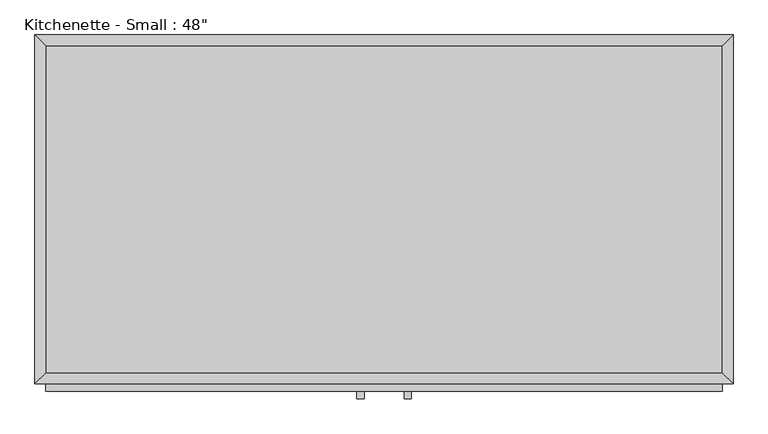
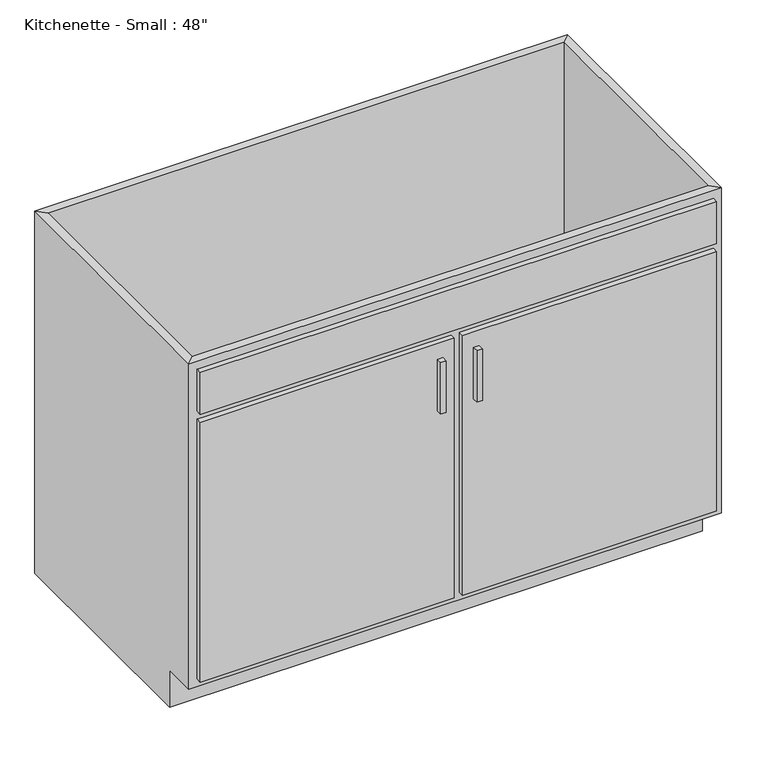
"""IFC4 building model written with IfcOpenShell, lengths in millimetres: proxy geometry."""

from ifc_helpers import new_model, si_unit, frame, origin, place, context, project, spatial, polyline, outline, extrude, faceted_brep, source, transform, mapped, element, save


def proxy_631763f9(model_context):
    return source(origin(), model_context, "Body", "SolidModel", [
        faceted_brep([(609.2877049, -590.55, 876.3), (609.2877049, -590.55, 88.9), (-571.8122951, -590.55, 88.9), (-571.8122951, -590.55, 876.3), (-590.8622951, -609.6, 876.3), (628.3377049, -609.6, 876.3), (-590.8622951, -609.6, 88.9), (628.3377049, -609.6, 88.9), (-571.8122951, -533.4, 88.9), (-571.8122951, -19.05, 88.9), (-571.8122951, -19.05, 876.3), (-590.8622951, 0.0, 876.3), (-590.8622951, 0.0, 0.0), (-590.8622951, -533.4, 0.0), (-590.8622951, -533.4, 88.9), (609.2877049, -19.05, 88.9), (609.2877049, -19.05, 876.3), (628.3377049, 0.0, 876.3), (628.3377049, 0.0, 0.0), (609.2877049, -533.4, 88.9), (628.3377049, -533.4, 88.9), (628.3377049, -533.4, 0.0)], [[[0, 1, 2, 3]], [[0, 3, 4, 5]], [[5, 4, 6, 7]], [[2, 1, 7, 6]], [[3, 2, 8, 9, 10]], [[4, 3, 10, 11]], [[6, 4, 11, 12, 13, 14]], [[2, 6, 14, 8]], [[10, 9, 15, 16]], [[11, 10, 16, 17]], [[12, 11, 17, 18]], [[1, 0, 16, 15, 19]], [[0, 5, 17, 16]], [[5, 7, 20, 21, 18, 17]], [[7, 1, 19, 20]], [[8, 19, 15, 9]], [[18, 21, 13, 12]], [[13, 21, 20, 19, 8, 14]]]),
        extrude(outline(polyline([(-16.1872951, -635.0), (-28.8872951, -635.0), (-28.8872951, -622.3), (-16.1872951, -622.3), (-16.1872951, -635.0)])), frame((0.0, 0.0, 573.769895), z_axis=(0.0, 0.0, 1.0), x_axis=(1.0, 0.0, 0.0)), (0.0, 0.0, 1.0), 124.730105),
        extrude(outline(polyline([(66.3627049, -635.0), (53.6627049, -635.0), (53.6627049, -622.3), (66.3627049, -622.3), (66.3627049, -635.0)])), frame((0.0, 0.0, 573.769895), z_axis=(0.0, 0.0, 1.0), x_axis=(1.0, 0.0, 0.0)), (0.0, 0.0, 1.0), 124.730105),
        extrude(outline(polyline([(609.2877049, -19.05), (609.2877049, -590.55), (-571.8122951, -590.55), (-571.8122951, -19.05), (609.2877049, -19.05)])), frame((0.0, 0.0, 88.9), z_axis=(0.0, 0.0, 1.0), x_axis=(1.0, 0.0, 0.0)), (0.0, 0.0, 1.0), 19.05),
        extrude(outline(polyline([(9.2127049, -622.3), (-571.8122951, -622.3), (-571.8122951, -609.6), (9.2127049, -609.6), (9.2127049, -622.3)])), frame((0.0, 0.0, 107.95), z_axis=(0.0, 0.0, 1.0), x_axis=(1.0, 0.0, 0.0)), (0.0, 0.0, 1.0), 628.65),
        extrude(outline(polyline([(609.2877049, -622.3), (28.2627049, -622.3), (28.2627049, -609.6), (609.2877049, -609.6), (609.2877049, -622.3)])), frame((0.0, 0.0, 107.95), z_axis=(0.0, 0.0, 1.0), x_axis=(1.0, 0.0, 0.0)), (0.0, 0.0, 1.0), 628.65),
        extrude(outline(polyline([(609.2877049, -622.3), (-571.8122951, -622.3), (-571.8122951, -609.6), (609.2877049, -609.6), (609.2877049, -622.3)])), frame((0.0, 0.0, 755.65), z_axis=(0.0, 0.0, 1.0), x_axis=(1.0, 0.0, 0.0)), (0.0, 0.0, 1.0), 101.6),
    ])


if __name__ == "__main__":
    model = new_model("IFC4")
    model_context = context("Model", 3, world=origin())
    ifc_project = project(units=[si_unit("LENGTHUNIT", "METRE", prefix="MILLI")], contexts=[model_context])
    site = spatial("IfcSite", under=ifc_project)
    building = spatial("IfcBuilding", under=site)
    placement = place(None, origin())
    proxy_shape = proxy_631763f9(model_context)
    element("IfcBuildingElementProxy", 1, Name="Kitchenette - Small : 48\"", ObjectType="Kitchenette - Small : 48\"", at=placement, inside=building, context=model_context, shape_type="MappedRepresentation", body=[
        mapped(proxy_shape, transform((0.0, 0.0, 0.0), x_axis=(1.0, 0.0, 0.0), y_axis=(0.0, 1.0, 0.0), z_axis=(0.0, 0.0, 1.0))),
    ])
    save(model, "model.ifc")

# Revit data of these elements
# Type "Kitchenette - Small : 48\""
#   Assembly Code = "E1090400"
#   Width = 4' - 0"
#   Height = 2' - 10 1/2"
#   Depth = 2' - 0"
#   Toe Depth = 0' - 3"
#   Toe Height = 0' - 3 1/2"
#   Cabinet Material = Cabinets
#   Door/Drawer Material = Cabinets
#   Handle Material = Cabinets - Handles
#   Default Elevation = 0
# Element 1 (IfcBuildingElementProxy, "Kitchenette - Small : 48\"")
#   Materials on its faces: "Cabinets", "Cabinets - Handles"
# Materials
#   "Cabinets": colour RGB 249 249 249, transparency 0
#   "Cabinets - Handles": class "Metal", colour RGB 57 57 57, transparency 0
